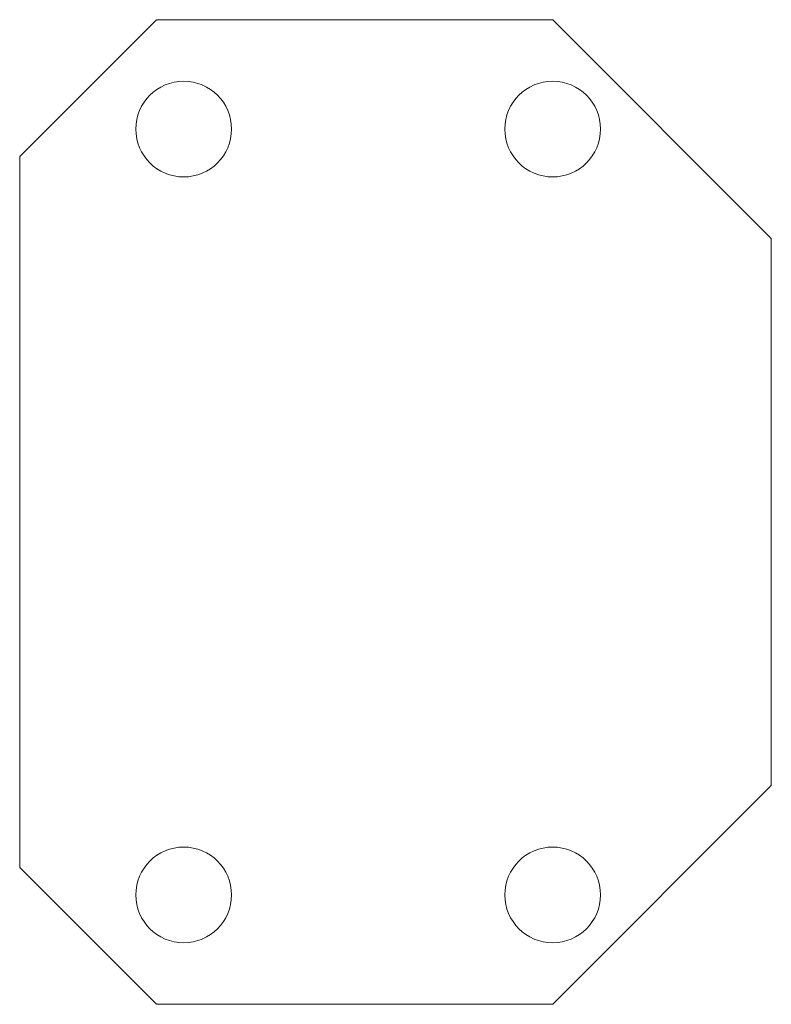
# Model space of a CAD drawing. Units: millimetres. Extents: x 400.5 to 455.5, y 767.3 to 839.3.
import ezdxf

# ---------------------------------------------------------------- set-up
doc = ezdxf.new("R2010")
doc.units = ezdxf.units.MM
doc.layers.add('M-CONS', color=8, linetype='Continuous', lineweight=18)

msp = doc.modelspace()

# ---------------------------------------------------------------- linework, layer by layer
at = {"layer": 'M-CONS'}
for p, q in [((400.478, 829.337), (410.478, 839.337)), ((439.478, 839.337), (410.478, 839.337)), ((439.478, 839.337), (455.478, 823.337)), ((400.478, 829.337), (400.478, 777.337)), ((455.478, 823.337), (455.478, 783.337)), ((439.478, 767.337), (455.478, 783.337)), ((400.478, 777.337), (410.478, 767.337)), ((410.478, 767.337), (439.478, 767.337))]:
    msp.add_line(p, q, dxfattribs=at)
for centre in [(412.478, 831.337), (439.478, 831.337), (412.478, 775.337), (439.478, 775.337)]:
    msp.add_circle(centre, 3.5, dxfattribs=at)

doc.saveas('drawing.dxf')
